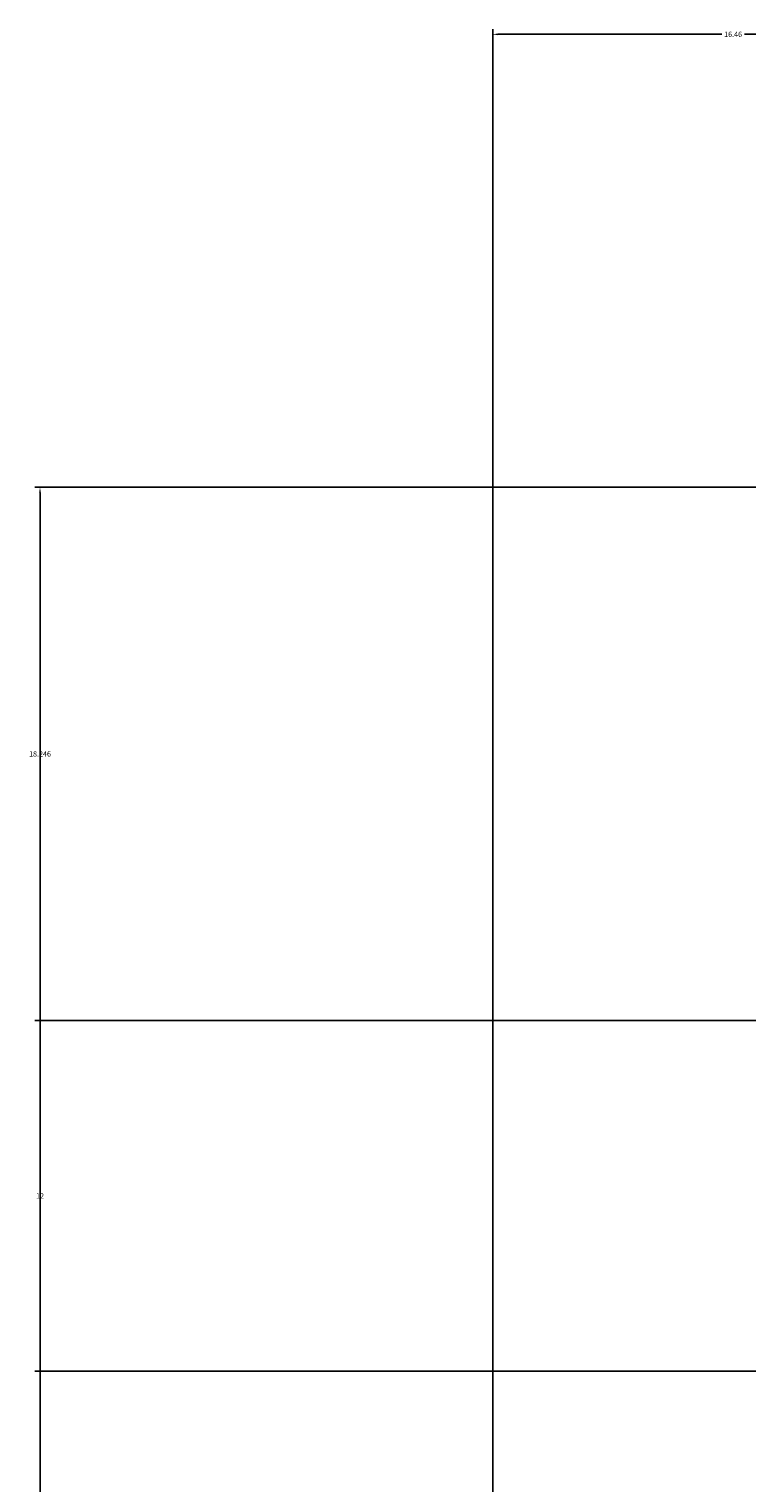
# Model space of a CAD drawing. Units: inches. Extents: x -6 to 289, y -8 to 323.
# Tile 44 of 107: x -6 to 19, y 273 to 323. Entities that reach past the tile are written whole.
import ezdxf

# ---------------------------------------------------------------- set-up
doc = ezdxf.new("R2010")
doc.units = ezdxf.units.IN
doc.header["$MEASUREMENT"] = 0
doc.layers.add('A-ANNO-DIMS', color=2, linetype='Continuous', lineweight=18)
doc.styles.get("Standard").update_dxf_attribs({"font": 'arial.ttf'})
doc.dimstyles.get("Standard").update_dxf_attribs({"dimtxt": 0.18, "dimasz": 0.18, "dimexe": 0.18, "dimexo": 0.0625, "dimgap": 0.09, "dimtad": 0, "dimtih": 1, "dimtoh": 1, "dimdec": 4, "dimzin": 0, "dimdsep": 46, "dimtxsty": 'Standard', "dimcen": 0.09, "dimadec": 0, "dimazin": 0, "dimtfac": 1, "dimtdec": 4, "dimtofl": 0, "dimtmove": 0, "dimatfit": 3, "dimfxl": 1, "dimtolj": 1, "dimtzin": 0, "dimarcsym": 0})

# ---------------------------------------------------------------- blocks, each defined once
blk = doc.blocks.new('*D19')
at = {"layer": 'A-ANNO-DIMS', "color": 0, "lineweight": -2, "transparency": 16777216}
for p, q in [((45.681, 277.043), (-5.737, 277.043)), ((-5.557, 276.863), (-5.557, 179.825)), ((-5.557, 82.423), (-5.557, 179.461)), ((45.681, 82.243), (-5.737, 82.243))]:
    blk.add_line(p, q, dxfattribs=at)
at = {"layer": 'A-ANNO-DIMS', "color": 0, "transparency": 16777216}
for points in [[(-5.587, 276.863), (-5.527, 276.863), (-5.557, 277.043)], [(-5.587, 82.423), (-5.527, 82.423), (-5.557, 82.243)]]:
    blk.add_solid(points, dxfattribs=at)
at = {"layer": 'Defpoints', "color": 0, "transparency": 16777216}
for p in [(-5.557, 277.043), (45.744, 277.043), (45.744, 82.243)]:
    blk.add_point(p, dxfattribs=at)
at = {"layer": 'A-ANNO-DIMS', "color": 0, "transparency": 16777216, "insert": (-5.557, 179.643), "char_height": 0.18, "attachment_point": 5}
blk.add_mtext('\\A1;194.8', dxfattribs=at)
blk = doc.blocks.new('*D20')
at = {"layer": 'A-ANNO-DIMS', "color": 0, "lineweight": -2, "transparency": 16777216}
for p, q in [((33.681, 289.043), (-5.737, 289.043)), ((-5.557, 288.863), (-5.557, 283.223)), ((-5.557, 277.223), (-5.557, 282.862)), ((45.681, 277.043), (-5.737, 277.043))]:
    blk.add_line(p, q, dxfattribs=at)
at = {"layer": 'A-ANNO-DIMS', "color": 0, "transparency": 16777216}
for points in [[(-5.587, 288.863), (-5.527, 288.863), (-5.557, 289.043)], [(-5.587, 277.223), (-5.527, 277.223), (-5.557, 277.043)]]:
    blk.add_solid(points, dxfattribs=at)
at = {"layer": 'Defpoints', "color": 0, "transparency": 16777216}
for p in [(-5.557, 289.043), (33.744, 289.043), (45.744, 277.043)]:
    blk.add_point(p, dxfattribs=at)
at = {"layer": 'A-ANNO-DIMS', "color": 0, "transparency": 16777216, "insert": (-5.557, 283.043), "char_height": 0.18, "attachment_point": 5}
blk.add_mtext('\\A1;12', dxfattribs=at)
blk = doc.blocks.new('*D21')
at = {"layer": 'A-ANNO-DIMS', "color": 0, "lineweight": -2, "transparency": 16777216}
for p, q in [((19.101, 307.289), (-5.737, 307.289)), ((-5.557, 307.109), (-5.557, 298.348)), ((-5.557, 289.223), (-5.557, 297.984)), ((33.681, 289.043), (-5.737, 289.043))]:
    blk.add_line(p, q, dxfattribs=at)
at = {"layer": 'A-ANNO-DIMS', "color": 0, "transparency": 16777216}
for points in [[(-5.587, 307.109), (-5.527, 307.109), (-5.557, 307.289)], [(-5.587, 289.223), (-5.527, 289.223), (-5.557, 289.043)]]:
    blk.add_solid(points, dxfattribs=at)
at = {"layer": 'Defpoints', "color": 0, "transparency": 16777216}
for p in [(-5.557, 307.289), (19.164, 307.289), (33.744, 289.043)]:
    blk.add_point(p, dxfattribs=at)
at = {"layer": 'A-ANNO-DIMS', "color": 0, "transparency": 16777216, "insert": (-5.557, 298.166), "char_height": 0.18, "attachment_point": 5}
blk.add_mtext('\\A1;18.246', dxfattribs=at)
blk = doc.blocks.new('*D22')
at = {"layer": 'A-ANNO-DIMS', "color": 0, "lineweight": -2, "transparency": 16777216}
for p, q in [((19.101, 307.289), (-5.737, 307.289)), ((-5.557, 307.109), (-5.557, 157.471)), ((-5.557, 7.469), (-5.557, 157.107)), ((11.907, 7.289), (-5.737, 7.289))]:
    blk.add_line(p, q, dxfattribs=at)
at = {"layer": 'A-ANNO-DIMS', "color": 0, "transparency": 16777216}
for points in [[(-5.587, 307.109), (-5.527, 307.109), (-5.557, 307.289)], [(-5.587, 7.469), (-5.527, 7.469), (-5.557, 7.289)]]:
    blk.add_solid(points, dxfattribs=at)
at = {"layer": 'Defpoints', "color": 0, "transparency": 16777216}
for p in [(19.164, 307.289), (-5.557, 7.289), (11.969, 7.289)]:
    blk.add_point(p, dxfattribs=at)
at = {"layer": 'A-ANNO-DIMS', "color": 0, "transparency": 16777216, "insert": (-5.557, 157.289), "char_height": 0.18, "attachment_point": 5}
blk.add_mtext('\\A1;300', dxfattribs=at)
blk = doc.blocks.new('*D57')
at = {"layer": 'A-ANNO-DIMS', "color": 0, "lineweight": -2, "transparency": 16777216}
for p, q in [((9.943, 68.495), (9.943, 322.969)), ((26.403, 68.495), (26.403, 322.969)), ((10.123, 322.789), (17.788, 322.789)), ((26.223, 322.789), (18.558, 322.789))]:
    blk.add_line(p, q, dxfattribs=at)
at = {"layer": 'A-ANNO-DIMS', "color": 0, "transparency": 16777216}
for points in [[(10.123, 322.819), (10.123, 322.759), (9.943, 322.789)], [(26.223, 322.819), (26.223, 322.759), (26.403, 322.789)]]:
    blk.add_solid(points, dxfattribs=at)
at = {"layer": 'Defpoints', "color": 0, "transparency": 16777216}
for p in [(26.403, 322.789), (9.943, 68.432), (26.403, 68.432)]:
    blk.add_point(p, dxfattribs=at)
at = {"layer": 'A-ANNO-DIMS', "color": 0, "transparency": 16777216, "insert": (18.173, 322.789), "char_height": 0.18, "attachment_point": 5}
blk.add_mtext('\\A1;16.46', dxfattribs=at)

msp = doc.modelspace()

# ---------------------------------------------------------------- dimensions: what is measured, and where the dimension line sits
at = {"layer": 'A-ANNO-DIMS'}
dim = msp.add_linear_dim(base=(26.403, 322.7888), p1=(9.943, 68.4322), p2=(26.403, 68.4322), dimstyle='Standard', override={"dimdec": 2, "dimlfac": 1, "dimrnd": 0, "dimzin": 0, "dimdsep": 46, "dimlunit": 2}, dxfattribs=at)
dim.commit()
dim.dimension.update_dxf_attribs({"geometry": '*D57', "text_midpoint": (18.173, 322.7888)})
for base, p1, p2, override, picture, middle in [((-5.557, 307.2888), (33.7437, 289.0427), (19.1638, 307.2888), {"dimdec": 3, "dimlfac": 1, "dimrnd": 0, "dimzin": 0, "dimdsep": 46, "dimlunit": 2}, '*D21', (-5.557, 298.1657)), ((-5.557, 7.2888), (19.1638, 307.2888), (11.9692, 7.2888), {"dimdec": 0, "dimlfac": 1, "dimrnd": 0, "dimzin": 0, "dimdsep": 46, "dimlunit": 2}, '*D22', (-5.557, 157.2888)), ((-5.557, 289.0427), (45.7437, 277.0427), (33.7437, 289.0427), {"dimdec": 0, "dimlfac": 1, "dimrnd": 0, "dimzin": 0, "dimdsep": 46, "dimlunit": 2}, '*D20', (-5.557, 283.0427)), ((-5.557, 277.0427), (45.7437, 82.2425), (45.7437, 277.0427), {"dimdec": 1, "dimlfac": 1, "dimrnd": 0, "dimzin": 0, "dimdsep": 46, "dimlunit": 2}, '*D19', (-5.557, 179.6426))]:
    dim = msp.add_linear_dim(base=base, p1=p1, p2=p2, angle=90, dimstyle='Standard', override=override, dxfattribs=at)
    dim.commit()
    dim.dimension.update_dxf_attribs({"geometry": picture, "text_midpoint": middle})

doc.saveas('drawing.dxf')
